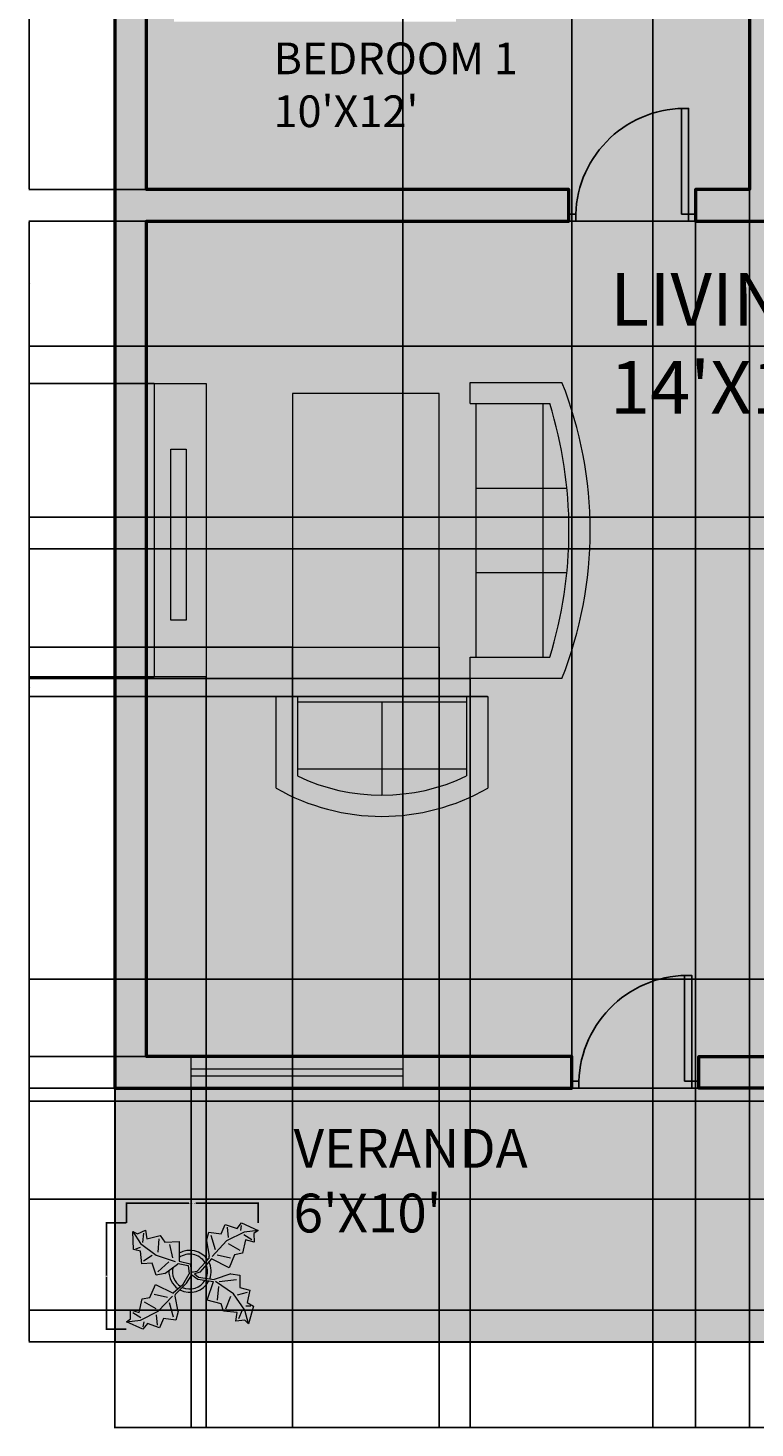
# Model space of a CAD drawing. Units: inches. Extents: x -494 to 1275, y 12 to 1194.
# Tile 1 of 8: x 87 to 293, y 346 to 743. Entities that reach past the tile are written whole.
import ezdxf

# ---------------------------------------------------------------- set-up
doc = ezdxf.new("R2010")
doc.units = ezdxf.units.IN
doc.header["$MEASUREMENT"] = 0
for name, color, linetype, lineweight in [('A-ANNO-DIMS', 2, 'Continuous', 18), ('A-AREA-IDEN', 7, 'Continuous', 25), ('A-DOOR', 3, 'Continuous', 25), ('A-DOOR-PATT', 7, 'Continuous', 13), ('A-FLOR', 7, 'Continuous', 30), ('A-FURN', 8, 'Continuous', 18), ('A-GLAZ', 4, 'Continuous', 18), ('A-GLAZ-FRAM-PATT', 7, 'Continuous', 13), ('A-GLAZ-GLAS-PATT', 4, 'Continuous', 13), ('A-WALL', 7, 'Continuous', 50), ('L-PLNT', 3, 'Continuous', 18)]:
    doc.layers.add(name, color=color, linetype=linetype, lineweight=lineweight)
for name, color, linetype, lineweight, true_color in [('A-FLOR-PATT', 51, 'Continuous', 13, 0xf8f6b0), ('A-FURN-PATT', 254, 'Continuous', 13, 0xfeeab9), ('A-WALL-PATT', 251, 'Continuous', 13, 0x636466)]:
    doc.layers.add(name, color=color, linetype=linetype, lineweight=lineweight, true_color=true_color)
doc.styles.get("Standard").update_dxf_attribs({"font": 'arial.ttf'})
doc.dimstyles.get("Standard").update_dxf_attribs({"dimtxt": 0.18, "dimasz": 0.18, "dimexe": 0.18, "dimexo": 0.0625, "dimgap": 0.09, "dimtad": 0, "dimtih": 1, "dimtoh": 1, "dimdec": 4, "dimzin": 0, "dimdsep": 46, "dimlunit": 4, "dimtxsty": 'Standard', "dimcen": 0.09, "dimadec": 0, "dimazin": 0, "dimtfac": 1, "dimtdec": 4, "dimtofl": 0, "dimtmove": 0, "dimatfit": 3, "dimfxl": 1, "dimtolj": 1, "dimtzin": 0, "dimarcsym": 0})

# ---------------------------------------------------------------- blocks, each defined once
blk = doc.blocks.new('Sofa - Roundback Loveseat 5 ft.')
for p, q in [((0, -32.44198), (0, -5.99998)), ((-24, -33.99998), (-24, -11.46958)), ((24.00004, -33.99998), (24.00004, -11.46958)), ((-23.9998, -13.38178), (23.99986, -13.38178)), ((-24, -32.44198), (24.00004, -32.44198))]:
    blk.add_line(p, q)
for points in [[(-24, -33.99998), (-30, -33.99998), (-30, -7.99998)], [(30.00004, -7.99998), (30.00004, -33.99998), (24.00004, -33.99998)]]:
    blk.add_lwpolyline(points)
for centre, radius, start, end in [((0, -60.24998), 60.24998, 60.13715, 119.8628), ((0, -61.38438), 55.38444, 64.32083, 115.6792)]:
    blk.add_arc(centre, radius, start, end)
blk = doc.blocks.new('WINDOW-60IN')
for p, q in [((3.5, 60), (3.5, 0)), ((5.5, 60), (5.5, 0))]:
    blk.add_line(p, q)
blk.add_lwpolyline([(9, 0), (0, 0), (0, 60), (9, 60)], close=True)
blk = doc.blocks.new('DOOR-SINGLE-36IN')
blk.add_lwpolyline([(34, 2, 0.414214), (2, 32), (4, 32), (4, 2), (2, 2), (2, 32)], format="xyb")
for points in [[(0, 0), (2, 0), (2, 2), (0, 2)], [(34, 0), (36, 0), (36, 2), (34, 2)]]:
    blk.add_lwpolyline(points, close=True)
blk = doc.blocks.new('PLANT-VERANDA')
h = blk.add_hatch(color=256)
h.dxf.hatch_style = 1
h.paths.add_polyline_path([(14.98, 24.96), (10.95, 24.77), (9.63, 26.57), (5.82, 25.7), (5.39, 28.16), (3.14, 27.06), (1.81, 27.74), (1.99, 22.6), (4, 22.14), (4.42, 18.56), (7.33, 18.76), (8.42, 15.4), (10.89, 15.82), (14.48, 18.48), (14.71, 18.7), (17.48, 18.06), (17.78, 15.71), (15.99, 12.65), (13.28, 10.22), (8.28, 12.71), (6.68, 9), (4.49, 8.6), (3.59, 4.8), (1.19, 5.49), (1.2, 2.99), (0, 2.09), (4.7, 0), (6, 1.6), (9.4, 0.41), (10.5, 3.11), (14, 2.62), (14.69, 5.02), (13.88, 9.42), (13.95, 9.99), (17.07, 13.11), (18.6, 15.45), (20.25, 14.18), (24.72, 13.6), (22.95, 8.3), (26.84, 7.24), (27.55, 5.12), (31.44, 4.77), (31.08, 2.29), (33.56, 2.64), (34.62, 1.58), (36.03, 6.53), (34.26, 7.59), (34.97, 11.13), (32.14, 11.84), (32.14, 15.37), (29.67, 15.73), (24.9, 14.15), (20.43, 14.8), (19.31, 15.71), (20.83, 16.24), (24.11, 19.95), (29.12, 17.46), (30.71, 21.17), (32.91, 21.57), (33.8, 25.37), (36.2, 24.68), (36.19, 27.18), (37.39, 28.08), (32.69, 30.17), (31.39, 28.57), (27.99, 29.76), (26.9, 27.06), (23.39, 27.55), (22.7, 25.15), (23.51, 20.75), (23.44, 20.18), (20.12, 16.5), (18.49, 16.24), (18.09, 18.58), (14.94, 19.37)])
h.paths.add_polyline_path([(14.94, 20.36), (14.94, 19.37), (18.09, 18.58), (18.49, 16.24), (20.12, 16.5), (22.33, 18.95, 0.422141)], flags=17)
h.paths.add_polyline_path([(17.78, 15.71), (17.48, 18.06), (14.71, 18.7), (14.48, 18.48), (13.15, 17.5, 0.320154), (15.44, 12.16), (15.99, 12.65)], flags=17)
h.paths.add_polyline_path([(22.35, 13.91), (20.25, 14.18), (18.6, 15.45), (17.07, 13.11), (15.85, 11.88, 0.365185)], flags=17)
h = blk.add_hatch(color=256)
h.dxf.hatch_style = 1
h.paths.add_polyline_path([(13.15, 17.5), (12.06, 16.69, 0.262498), (14.67, 11.47), (15.44, 12.16, -0.320272)])
h.paths.add_polyline_path([(14.95, 21.58), (14.94, 19.37), (18.09, 18.58), (18.49, 16.24), (20.12, 16.5), (23.05, 19.75, 0.39032)])
h = blk.add_hatch(color=256)
h.dxf.hatch_style = 1
h.paths.add_polyline_path([(22.65, 18.29), (20.83, 16.24), (19.31, 15.71), (20.43, 14.8), (22.64, 14.48, 0.196749)])
h.paths.add_polyline_path([(23.39, 19.14), (22.65, 18.29, -0.196749), (22.64, 14.48), (23.64, 14.33, 0.213013)])
h.paths.add_polyline_path([(23.41, 13.77), (20.25, 14.18), (18.6, 15.45), (17.07, 13.11), (15.15, 11.19, 0.412433)])
for p, q in [((3.14, 27.06), (5.39, 28.16)), ((5.39, 28.16), (5.82, 25.7)), ((26.9, 27.06), (27.99, 29.76)), ((27.99, 29.76), (31.39, 28.57)), ((28.59, 28.96), (28.9, 26.06)), ((31.39, 28.57), (32.69, 30.17)), ((32.59, 29.47), (32.39, 28.07)), ((32.69, 30.17), (37.39, 28.08)), ((37.39, 28.08), (33.39, 27.57)), ((37.39, 28.08), (36.19, 27.18)), ((1.81, 27.74), (4.02, 24.37)), ((1.81, 27.74), (3.14, 27.06)), ((1.99, 22.6), (1.81, 27.74)), ((4.02, 24.37), (8.46, 20.99)), ((4.69, 24.59), (4.93, 27.27)), ((5.82, 25.7), (9.63, 26.57)), ((9.17, 25.68), (8.92, 21.88)), ((9.63, 26.57), (10.95, 24.77)), ((10.95, 24.77), (14.98, 24.96)), ((13.16, 20.28), (12.29, 24.09)), ((14.98, 24.96), (14.94, 19.37)), ((22.7, 25.15), (23.39, 27.55)), ((22.7, 25.15), (23.51, 20.75)), ((23.39, 27.55), (26.9, 27.06)), ((24, 26.75), (25.21, 22.65)), ((28.4, 25.06), (24.29, 20.67)), ((33.39, 27.57), (28.4, 25.06)), ((32.31, 22.37), (29, 24.26)), ((33.8, 25.37), (32.91, 21.57)), ((33.3, 26.87), (35.6, 25.48)), ((36.2, 24.68), (33.8, 25.37)), ((36.19, 27.18), (36.2, 24.68)), ((4, 22.14), (1.99, 22.6)), ((2.66, 22.82), (4.01, 23.26)), ((4.42, 18.56), (4, 22.14)), ((4.88, 19.45), (7.35, 20.99)), ((8.46, 20.99), (13.82, 19.26)), ((20.12, 16.5), (23.44, 20.18)), ((24.11, 19.95), (20.83, 16.24)), ((23.44, 20.18), (23.51, 20.75)), ((29.12, 17.46), (24.11, 19.95)), ((25.71, 21.16), (29.51, 20.26)), ((30.71, 21.17), (29.12, 17.46)), ((32.91, 21.57), (30.71, 21.17)), ((7.33, 18.76), (4.42, 18.56)), ((8.42, 15.4), (7.33, 18.76)), ((8.88, 16.29), (12.03, 19.17)), ((10.89, 15.82), (14.48, 18.48)), ((14.48, 18.48), (14.71, 18.7)), ((14.71, 18.7), (17.48, 18.06)), ((14.94, 19.37), (18.09, 18.58)), ((17.48, 18.06), (17.78, 15.71)), ((17.48, 18.06), (17.48, 18.06)), ((18.09, 18.58), (18.49, 16.24)), ((18.49, 16.24), (20.12, 16.5)), ((20.83, 16.24), (19.31, 15.71)), ((6.68, 9), (8.28, 12.71)), ((8.28, 12.71), (13.28, 10.22)), ((10.89, 15.82), (8.42, 15.4)), ((15.99, 12.65), (13.28, 10.22)), ((13.95, 9.99), (17.07, 13.11)), ((15.99, 12.65), (17.78, 15.71)), ((17.07, 13.11), (18.6, 15.45)), ((18.6, 15.45), (20.25, 14.18)), ((19.31, 15.71), (20.43, 14.8)), ((20.25, 14.18), (24.72, 13.6)), ((20.43, 14.8), (24.9, 14.15)), ((22.95, 8.3), (24.72, 13.6)), ((29.67, 15.73), (24.9, 14.15)), ((30.38, 10.07), (25.23, 13.59)), ((26.13, 12.19), (25.78, 8.3)), ((26.36, 13.52), (31.21, 14.1)), ((29.67, 15.73), (32.14, 15.37)), ((32.14, 15.37), (32.14, 11.84)), ((3.59, 4.8), (4.49, 8.6)), ((4.49, 8.6), (6.68, 9)), ((11.68, 9.02), (7.88, 9.91)), ((8.99, 5.11), (13.1, 9.45)), ((13.88, 9.42), (13.95, 9.99)), ((14.69, 5.02), (13.88, 9.42)), ((26.84, 7.24), (22.95, 8.3)), ((28.25, 5.83), (29.67, 9.36)), ((33.56, 5.47), (30.38, 10.07)), ((34.26, 10.42), (31.44, 9.72)), ((32.14, 11.84), (34.97, 11.13)), ((34.97, 11.13), (34.26, 7.59)), ((1.19, 5.49), (3.59, 4.8)), ((1.2, 2.99), (1.19, 5.49)), ((4.1, 3.3), (1.79, 4.69)), ((4, 2.6), (8.99, 5.11)), ((5.09, 7.8), (8.39, 5.91)), ((8.8, 1.21), (8.5, 4.11)), ((13.4, 3.42), (12.19, 7.52)), ((14.69, 5.02), (14, 2.62)), ((27.55, 5.12), (26.84, 7.24)), ((31.44, 4.77), (27.55, 5.12)), ((31.08, 2.29), (31.44, 4.77)), ((32.85, 5.47), (31.79, 3)), ((34.62, 1.58), (33.56, 5.47)), ((35.33, 6.53), (33.91, 6.53)), ((34.26, 7.59), (36.03, 6.53)), ((36.03, 6.53), (34.62, 1.58)), ((0, 2.09), (1.2, 2.99)), ((0, 2.09), (4, 2.6)), ((4.7, 0), (0, 2.09)), ((6, 1.6), (4.7, 0)), ((4.8, 0.7), (5, 2.1)), ((9.4, 0.41), (6, 1.6)), ((10.5, 3.11), (9.4, 0.41)), ((14, 2.62), (10.5, 3.11)), ((33.56, 2.64), (31.08, 2.29)), ((34.62, 1.58), (33.56, 2.64))]:
    blk.add_line(p, q)
for centre, radius, start, end in [((18.01, 16.27), 6.13, 34.3757, 120.1028), ((17.95, 16.06), 5.25, 33.8219, 124.9414), ((18, 16.4), 5.94, 177.1741, 236.0068), ((18.04, 16.43), 5, 167.6804, 238.6774), ((17.99, 16.39), 5.03, 337.6469, 22.1698), ((18.14, 16.45), 5.9, 338.9388, 27.0389), ((17.98, 16.63), 6.14, 242.5292, 332.1842), ((17.9, 16.76), 5.29, 247.3711, 327.472)]:
    blk.add_arc(centre, radius, start, end)
blk = doc.blocks.new('SOFA-84IN-PLAN')
h = blk.add_hatch(color=256)
h.dxf.hatch_style = 1
h.paths.add_polyline_path([(20.62, 54), (1.56, 54), (1.56, 30), (20.62, 30)], flags=17)
h.paths.add_polyline_path([(20.62, 78), (1.56, 78), (1.56, 54), (20.62, 54)], flags=17)
h.paths.add_polyline_path([(22.53, 78), (20.62, 78), (20.62, 54), (27.4, 54, 0.050647)], flags=17)
h.paths.add_polyline_path([(27.4, 54), (20.62, 54), (20.62, 30), (27.4, 30, 0.049628)], flags=17)
h.paths.add_polyline_path([(20.62, 30), (1.56, 30), (1.56, 6), (20.62, 6)], flags=17)
h.paths.add_polyline_path([(27.4, 30), (20.62, 30), (20.62, 6), (22.53, 6, 0.050647)], flags=17)
h.paths.add_polyline_path([(26, 84), (0, 84), (0, 78), (22.53, 78, -0.050647), (27.4, 54, -0.100528), (22.53, 6), (20.62, 6), (1.56, 6), (0, 6), (0, 0), (26, 0, 0.190476)])
for p, q in [((0, 78), (22.53, 78)), ((1.56, 78), (1.56, 6)), ((20.62, 78), (20.62, 6)), ((1.56, 54), (27.4, 54)), ((1.56, 30), (27.4, 30)), ((0, 6), (22.53, 6))]:
    blk.add_line(p, q)
for points in [[(0, 78), (0, 84), (26, 84)], [(26, 0), (0, 0), (0, 6)]]:
    blk.add_lwpolyline(points)
for centre, radius, start, end in [((-80.25, 42), 114.25, 338.4314, 21.5686), ((-93.2, 42), 121.2, 342.7203, 17.2797)]:
    blk.add_arc(centre, radius, start, end)
blk = doc.blocks.new('TABLE-RECTANGULAR-72IN')
h = blk.add_hatch(color=256)
h.dxf.hatch_style = 1
h.paths.add_polyline_path([(41.56, 71.99), (0, 71.99), (0, 0), (41.56, 0)])
blk.add_lwpolyline([(0, 0), (41.56, 0), (41.56, 71.99), (0, 71.99)], close=True)
blk = doc.blocks.new('MEDIA-CONSOLE-PLAN')
for p, q in [((4.67, 64.59), (9.03, 64.59)), ((4.67, 16.07), (4.67, 64.59)), ((9.03, 64.59), (9.03, 16.07)), ((9.03, 16.07), (4.67, 16.07))]:
    blk.add_line(p, q)
blk.add_lwpolyline([(0, 83.25), (14.68, 83.25), (14.68, 0), (0, 0)], close=True)
blk = doc.blocks.new('*D30')
at = {"layer": 'A-ANNO-DIMS', "color": 0, "lineweight": -2, "transparency": 16777216}
for p, q in [((115.01, 404.34), (115.01, 410.07)), ((115.19, 409.89), (132.74, 409.89)), ((152.22, 409.89), (134.67, 409.89)), ((152.4, 404.34), (152.4, 410.07))]:
    blk.add_line(p, q, dxfattribs=at)
at = {"layer": 'A-ANNO-DIMS', "color": 0, "transparency": 16777216}
for points in [[(115.19, 409.92), (115.19, 409.86), (115.01, 409.89)], [(152.22, 409.92), (152.22, 409.86), (152.4, 409.89)]]:
    blk.add_solid(points, dxfattribs=at)
at = {"layer": 'Defpoints', "color": 0, "transparency": 16777216}
for p in [(152.4, 409.89), (115.01, 404.28), (152.4, 404.28)]:
    blk.add_point(p, dxfattribs=at)
at = {"layer": 'A-ANNO-DIMS', "color": 0, "transparency": 16777216, "insert": (133.7, 409.89), "char_height": 0.18, "attachment_point": 5}
blk.add_mtext('\\A1;PLANT 37 TYP.', dxfattribs=at)
blk = doc.blocks.new('*D31')
at = {"layer": 'A-ANNO-DIMS', "color": 0, "lineweight": -2, "transparency": 16777216}
for p, q in [((114.94, 404.28), (109.22, 404.28)), ((109.4, 404.1), (109.4, 389.38)), ((109.4, 374.29), (109.4, 389.01)), ((114.94, 374.11), (109.22, 374.11))]:
    blk.add_line(p, q, dxfattribs=at)
at = {"layer": 'A-ANNO-DIMS', "color": 0, "transparency": 16777216}
for points in [[(109.37, 404.1), (109.43, 404.1), (109.4, 404.28)], [(109.37, 374.29), (109.43, 374.29), (109.4, 374.11)]]:
    blk.add_solid(points, dxfattribs=at)
at = {"layer": 'Defpoints', "color": 0, "transparency": 16777216}
for p in [(109.4, 404.28), (115.01, 404.28), (115.01, 374.11)]:
    blk.add_point(p, dxfattribs=at)
at = {"layer": 'A-ANNO-DIMS', "color": 0, "transparency": 16777216, "insert": (109.4, 389.2), "char_height": 0.18, "attachment_point": 5}
blk.add_mtext('\\A1;30 TYP.', dxfattribs=at)
blk = doc.blocks.new('*D42')
at = {"layer": 'A-ANNO-DIMS', "color": 0, "lineweight": -2, "transparency": 16777216}
for p, q in [((111.73, 370.47), (111.73, 346.1)), ((471.73, 370.47), (471.73, 346.1)), ((111.91, 346.28), (291.44, 346.28)), ((471.55, 346.28), (292.02, 346.28))]:
    blk.add_line(p, q, dxfattribs=at)
at = {"layer": 'A-ANNO-DIMS', "color": 0, "transparency": 16777216}
for points in [[(111.91, 346.31), (111.91, 346.25), (111.73, 346.28)], [(471.55, 346.31), (471.55, 346.25), (471.73, 346.28)]]:
    blk.add_solid(points, dxfattribs=at)
at = {"layer": 'Defpoints', "color": 0, "transparency": 16777216}
for p in [(111.73, 370.53), (471.73, 370.53), (471.73, 346.28)]:
    blk.add_point(p, dxfattribs=at)
at = {"layer": 'A-ANNO-DIMS', "color": 0, "transparency": 16777216, "insert": (291.73, 346.28), "char_height": 0.18, "attachment_point": 5}
blk.add_mtext('\\A1;360', dxfattribs=at)
blk = doc.blocks.new('*D44')
at = {"layer": 'A-ANNO-DIMS', "color": 0, "lineweight": -2, "transparency": 16777216}
for p, q in [((111.67, 442.53), (87.3, 442.53)), ((87.48, 442.35), (87.48, 406.72)), ((87.48, 370.71), (87.48, 406.35)), ((111.67, 370.53), (87.3, 370.53))]:
    blk.add_line(p, q, dxfattribs=at)
at = {"layer": 'A-ANNO-DIMS', "color": 0, "transparency": 16777216}
for points in [[(87.45, 442.35), (87.51, 442.35), (87.48, 442.53)], [(87.45, 370.71), (87.51, 370.71), (87.48, 370.53)]]:
    blk.add_solid(points, dxfattribs=at)
at = {"layer": 'Defpoints', "color": 0, "transparency": 16777216}
for p in [(87.48, 442.53), (111.73, 442.53), (111.73, 370.53)]:
    blk.add_point(p, dxfattribs=at)
at = {"layer": 'A-ANNO-DIMS', "color": 0, "transparency": 16777216, "insert": (87.48, 406.53), "char_height": 0.18, "attachment_point": 5}
blk.add_mtext('\\A1;72', dxfattribs=at)
blk = doc.blocks.new('*D45')
at = {"layer": 'A-ANNO-DIMS', "color": 0, "lineweight": -2, "transparency": 16777216}
for p, q in [((120.67, 841.53), (87.3, 841.53)), ((87.48, 841.35), (87.48, 769.72)), ((87.48, 697.71), (87.48, 769.35)), ((120.67, 697.53), (87.3, 697.53))]:
    blk.add_line(p, q, dxfattribs=at)
at = {"layer": 'A-ANNO-DIMS', "color": 0, "transparency": 16777216}
for points in [[(87.45, 841.35), (87.51, 841.35), (87.48, 841.53)], [(87.45, 697.71), (87.51, 697.71), (87.48, 697.53)]]:
    blk.add_solid(points, dxfattribs=at)
at = {"layer": 'Defpoints', "color": 0, "transparency": 16777216}
for p in [(120.73, 841.53), (87.48, 697.53), (120.73, 697.53)]:
    blk.add_point(p, dxfattribs=at)
at = {"layer": 'A-ANNO-DIMS', "color": 0, "transparency": 16777216, "insert": (87.48, 769.53), "char_height": 0.18, "attachment_point": 5}
blk.add_mtext('\\A1;144', dxfattribs=at)
blk = doc.blocks.new('*D46')
at = {"layer": 'A-ANNO-DIMS', "color": 0, "lineweight": -2, "transparency": 16777216}
for p, q in [((120.67, 688.53), (87.3, 688.53)), ((87.48, 688.35), (87.48, 570.22)), ((87.48, 451.71), (87.48, 569.85)), ((120.67, 451.53), (87.3, 451.53))]:
    blk.add_line(p, q, dxfattribs=at)
at = {"layer": 'A-ANNO-DIMS', "color": 0, "transparency": 16777216}
for points in [[(87.45, 688.35), (87.51, 688.35), (87.48, 688.53)], [(87.45, 451.71), (87.51, 451.71), (87.48, 451.53)]]:
    blk.add_solid(points, dxfattribs=at)
at = {"layer": 'Defpoints', "color": 0, "transparency": 16777216}
for p in [(87.48, 688.53), (120.73, 688.53), (120.73, 451.53)]:
    blk.add_point(p, dxfattribs=at)
at = {"layer": 'A-ANNO-DIMS', "color": 0, "transparency": 16777216, "insert": (87.48, 570.03), "char_height": 0.18, "attachment_point": 5}
blk.add_mtext('\\A1;237', dxfattribs=at)
blk = doc.blocks.new('*D51')
at = {"layer": 'A-ANNO-DIMS', "color": 0, "lineweight": -2, "transparency": 16777216}
for p, q in [((111.73, 442.47), (111.73, 346.1)), ((133.38, 442.47), (133.38, 346.1)), ((111.91, 346.28), (122.09, 346.28)), ((133.2, 346.28), (123.02, 346.28))]:
    blk.add_line(p, q, dxfattribs=at)
at = {"layer": 'A-ANNO-DIMS', "color": 0, "transparency": 16777216}
for points in [[(111.91, 346.31), (111.91, 346.25), (111.73, 346.28)], [(133.2, 346.31), (133.2, 346.25), (133.38, 346.28)]]:
    blk.add_solid(points, dxfattribs=at)
at = {"layer": 'Defpoints', "color": 0, "transparency": 16777216}
for p in [(111.73, 442.53), (133.38, 442.53), (133.38, 346.28)]:
    blk.add_point(p, dxfattribs=at)
at = {"layer": 'A-ANNO-DIMS', "color": 0, "transparency": 16777216, "insert": (122.56, 346.28), "char_height": 0.18, "attachment_point": 5}
blk.add_mtext('\\A1;21.646', dxfattribs=at)
blk = doc.blocks.new('*D52')
at = {"layer": 'A-ANNO-DIMS', "color": 0, "lineweight": -2, "transparency": 16777216}
for p, q in [((193.38, 451.6), (193.38, 874.96)), ((193.56, 874.78), (216.96, 874.78)), ((241.16, 874.78), (217.76, 874.78)), ((241.34, 451.6), (241.34, 874.96))]:
    blk.add_line(p, q, dxfattribs=at)
at = {"layer": 'A-ANNO-DIMS', "color": 0, "transparency": 16777216}
for points in [[(193.56, 874.81), (193.56, 874.75), (193.38, 874.78)], [(241.16, 874.81), (241.16, 874.75), (241.34, 874.78)]]:
    blk.add_solid(points, dxfattribs=at)
at = {"layer": 'Defpoints', "color": 0, "transparency": 16777216}
for p in [(241.34, 874.78), (193.38, 451.53), (241.34, 451.53)]:
    blk.add_point(p, dxfattribs=at)
at = {"layer": 'A-ANNO-DIMS', "color": 0, "transparency": 16777216, "insert": (217.36, 874.78), "char_height": 0.18, "attachment_point": 5}
blk.add_mtext('\\A1;47.96', dxfattribs=at)
blk = doc.blocks.new('*D54')
at = {"layer": 'A-ANNO-DIMS', "color": 0, "lineweight": -2, "transparency": 16777216}
for p, q in [((291.73, 697.47), (291.73, 346.1)), ((276.46, 688.47), (276.46, 346.1)), ((276.64, 346.28), (283.64, 346.28)), ((291.55, 346.28), (284.55, 346.28))]:
    blk.add_line(p, q, dxfattribs=at)
at = {"layer": 'A-ANNO-DIMS', "color": 0, "transparency": 16777216}
for points in [[(276.64, 346.31), (276.64, 346.25), (276.46, 346.28)], [(291.55, 346.31), (291.55, 346.25), (291.73, 346.28)]]:
    blk.add_solid(points, dxfattribs=at)
at = {"layer": 'Defpoints', "color": 0, "transparency": 16777216}
for p in [(291.73, 697.53), (276.46, 688.53), (291.73, 346.28)]:
    blk.add_point(p, dxfattribs=at)
at = {"layer": 'A-ANNO-DIMS', "color": 0, "transparency": 16777216, "insert": (284.09, 346.28), "char_height": 0.18, "attachment_point": 5}
blk.add_mtext('\\A1;15.276', dxfattribs=at)
blk = doc.blocks.new('*D55')
at = {"layer": 'A-ANNO-DIMS', "color": 0, "lineweight": -2, "transparency": 16777216}
for p, q in [((402.67, 688.53), (87.3, 688.53)), ((87.48, 688.35), (87.48, 646.72)), ((87.48, 604.71), (87.48, 646.35)), ((402.67, 604.53), (87.3, 604.53))]:
    blk.add_line(p, q, dxfattribs=at)
at = {"layer": 'A-ANNO-DIMS', "color": 0, "transparency": 16777216}
for points in [[(87.45, 688.35), (87.51, 688.35), (87.48, 688.53)], [(87.45, 604.71), (87.51, 604.71), (87.48, 604.53)]]:
    blk.add_solid(points, dxfattribs=at)
at = {"layer": 'Defpoints', "color": 0, "transparency": 16777216}
for p in [(87.48, 688.53), (402.73, 688.53), (402.73, 604.53)]:
    blk.add_point(p, dxfattribs=at)
at = {"layer": 'A-ANNO-DIMS', "color": 0, "transparency": 16777216, "insert": (87.48, 646.53), "char_height": 0.18, "attachment_point": 5}
blk.add_mtext('\\A1;84', dxfattribs=at)
blk = doc.blocks.new('*D59')
at = {"layer": 'A-ANNO-DIMS', "color": 0, "lineweight": -2, "transparency": 16777216}
for p, q in [((342.67, 473.5), (87.3, 473.5)), ((87.48, 473.32), (87.48, 426.7)), ((87.48, 379.71), (87.48, 426.33)), ((342.67, 379.53), (87.3, 379.53))]:
    blk.add_line(p, q, dxfattribs=at)
at = {"layer": 'A-ANNO-DIMS', "color": 0, "transparency": 16777216}
for points in [[(87.45, 473.32), (87.51, 473.32), (87.48, 473.5)], [(87.45, 379.71), (87.51, 379.71), (87.48, 379.53)]]:
    blk.add_solid(points, dxfattribs=at)
at = {"layer": 'Defpoints', "color": 0, "transparency": 16777216}
for p in [(87.48, 473.5), (342.73, 473.5), (342.73, 379.53)]:
    blk.add_point(p, dxfattribs=at)
at = {"layer": 'A-ANNO-DIMS', "color": 0, "transparency": 16777216, "insert": (87.48, 426.52), "char_height": 0.18, "attachment_point": 5}
blk.add_mtext('\\A1;93.96', dxfattribs=at)
blk = doc.blocks.new('*D61')
at = {"layer": 'A-ANNO-DIMS', "color": 0, "lineweight": -2, "transparency": 16777216}
for p, q in [((393.67, 688.53), (87.3, 688.53)), ((87.48, 688.35), (87.48, 671.01)), ((87.48, 653.3), (87.48, 670.64)), ((393.67, 653.12), (87.3, 653.12))]:
    blk.add_line(p, q, dxfattribs=at)
at = {"layer": 'A-ANNO-DIMS', "color": 0, "transparency": 16777216}
for points in [[(87.45, 688.35), (87.51, 688.35), (87.48, 688.53)], [(87.45, 653.3), (87.51, 653.3), (87.48, 653.12)]]:
    blk.add_solid(points, dxfattribs=at)
at = {"layer": 'Defpoints', "color": 0, "transparency": 16777216}
for p in [(393.73, 688.53), (87.48, 653.12), (393.73, 653.12)]:
    blk.add_point(p, dxfattribs=at)
at = {"layer": 'A-ANNO-DIMS', "color": 0, "transparency": 16777216, "insert": (87.48, 670.83), "char_height": 0.18, "attachment_point": 5}
blk.add_mtext('\\A1;35.416', dxfattribs=at)
blk = doc.blocks.new('*D63')
at = {"layer": 'A-ANNO-DIMS', "color": 0, "lineweight": -2, "transparency": 16777216}
for p, q in [((402.67, 595.53), (87.3, 595.53)), ((87.48, 595.35), (87.48, 487.72)), ((87.48, 379.71), (87.48, 487.35)), ((342.67, 379.53), (87.3, 379.53))]:
    blk.add_line(p, q, dxfattribs=at)
at = {"layer": 'A-ANNO-DIMS', "color": 0, "transparency": 16777216}
for points in [[(87.45, 595.35), (87.51, 595.35), (87.48, 595.53)], [(87.45, 379.71), (87.51, 379.71), (87.48, 379.53)]]:
    blk.add_solid(points, dxfattribs=at)
at = {"layer": 'Defpoints', "color": 0, "transparency": 16777216}
for p in [(402.73, 595.53), (87.48, 379.53), (342.73, 379.53)]:
    blk.add_point(p, dxfattribs=at)
at = {"layer": 'A-ANNO-DIMS', "color": 0, "transparency": 16777216, "insert": (87.48, 487.53), "char_height": 0.18, "attachment_point": 5}
blk.add_mtext('\\A1;216', dxfattribs=at)
blk = doc.blocks.new('*D68')
at = {"layer": 'A-ANNO-DIMS', "color": 0, "lineweight": -2, "transparency": 16777216}
for p, q in [((458.91, 438.82), (87.3, 438.82)), ((87.48, 438.64), (87.48, 409.36)), ((87.48, 379.71), (87.48, 408.99)), ((462.68, 379.53), (87.3, 379.53))]:
    blk.add_line(p, q, dxfattribs=at)
at = {"layer": 'A-ANNO-DIMS', "color": 0, "transparency": 16777216}
for points in [[(87.45, 438.64), (87.51, 438.64), (87.48, 438.82)], [(87.45, 379.71), (87.51, 379.71), (87.48, 379.53)]]:
    blk.add_solid(points, dxfattribs=at)
at = {"layer": 'Defpoints', "color": 0, "transparency": 16777216}
for p in [(87.48, 438.82), (458.98, 438.82), (462.74, 379.53)]:
    blk.add_point(p, dxfattribs=at)
at = {"layer": 'A-ANNO-DIMS', "color": 0, "transparency": 16777216, "insert": (87.48, 409.18), "char_height": 0.18, "attachment_point": 5}
blk.add_mtext('\\A1;59.28', dxfattribs=at)
blk = doc.blocks.new('*D82')
at = {"layer": 'A-ANNO-DIMS', "color": 0, "lineweight": -2, "transparency": 16777216}
for p, q in [((264.34, 820.48), (264.34, 346.1)), ((291.73, 820.48), (291.73, 346.1)), ((264.52, 346.28), (277.57, 346.28)), ((291.55, 346.28), (278.5, 346.28))]:
    blk.add_line(p, q, dxfattribs=at)
at = {"layer": 'A-ANNO-DIMS', "color": 0, "transparency": 16777216}
for points in [[(264.52, 346.31), (264.52, 346.25), (264.34, 346.28)], [(291.55, 346.31), (291.55, 346.25), (291.73, 346.28)]]:
    blk.add_solid(points, dxfattribs=at)
at = {"layer": 'Defpoints', "color": 0, "transparency": 16777216}
for p in [(264.34, 820.54), (291.73, 820.54), (291.73, 346.28)]:
    blk.add_point(p, dxfattribs=at)
at = {"layer": 'A-ANNO-DIMS', "color": 0, "transparency": 16777216, "insert": (278.04, 346.28), "char_height": 0.18, "attachment_point": 5}
blk.add_mtext('\\A1;27.394', dxfattribs=at)
blk = doc.blocks.new('*D86')
at = {"layer": 'A-ANNO-DIMS', "color": 0, "lineweight": -2, "transparency": 16777216}
for p, q in [((120.67, 688.53), (87.3, 688.53)), ((87.48, 688.35), (87.48, 665.71)), ((87.48, 642.7), (87.48, 665.34)), ((122.89, 642.52), (87.3, 642.52))]:
    blk.add_line(p, q, dxfattribs=at)
at = {"layer": 'A-ANNO-DIMS', "color": 0, "transparency": 16777216}
for points in [[(87.45, 688.35), (87.51, 688.35), (87.48, 688.53)], [(87.45, 642.7), (87.51, 642.7), (87.48, 642.52)]]:
    blk.add_solid(points, dxfattribs=at)
at = {"layer": 'Defpoints', "color": 0, "transparency": 16777216}
for p in [(120.73, 688.53), (87.48, 642.52), (122.96, 642.52)]:
    blk.add_point(p, dxfattribs=at)
at = {"layer": 'A-ANNO-DIMS', "color": 0, "transparency": 16777216, "insert": (87.48, 665.53), "char_height": 0.18, "attachment_point": 5}
blk.add_mtext('\\A1;46.02', dxfattribs=at)
blk = doc.blocks.new('*D87')
at = {"layer": 'A-ANNO-DIMS', "color": 0, "lineweight": -2, "transparency": 16777216}
for p, q in [((162.13, 567.63), (162.13, 346.1)), ((137.63, 559.21), (137.63, 346.1)), ((137.81, 346.28), (149.48, 346.28)), ((161.95, 346.28), (150.28, 346.28))]:
    blk.add_line(p, q, dxfattribs=at)
at = {"layer": 'A-ANNO-DIMS', "color": 0, "transparency": 16777216}
for points in [[(137.81, 346.31), (137.81, 346.25), (137.63, 346.28)], [(161.95, 346.31), (161.95, 346.25), (162.13, 346.28)]]:
    blk.add_solid(points, dxfattribs=at)
at = {"layer": 'Defpoints', "color": 0, "transparency": 16777216}
for p in [(162.13, 567.7), (137.63, 559.27), (162.13, 346.28)]:
    blk.add_point(p, dxfattribs=at)
at = {"layer": 'A-ANNO-DIMS', "color": 0, "transparency": 16777216, "insert": (149.88, 346.28), "char_height": 0.18, "attachment_point": 5}
blk.add_mtext('\\A1;24.49', dxfattribs=at)
blk = doc.blocks.new('*D88')
at = {"layer": 'A-ANNO-DIMS', "color": 0, "lineweight": -2, "transparency": 16777216}
for p, q in [((203.69, 567.63), (203.69, 346.1)), ((212.54, 558.75), (212.54, 346.1)), ((203.87, 346.28), (207.72, 346.28)), ((212.36, 346.28), (208.51, 346.28))]:
    blk.add_line(p, q, dxfattribs=at)
at = {"layer": 'A-ANNO-DIMS', "color": 0, "transparency": 16777216}
for points in [[(203.87, 346.31), (203.87, 346.25), (203.69, 346.28)], [(212.36, 346.31), (212.36, 346.25), (212.54, 346.28)]]:
    blk.add_solid(points, dxfattribs=at)
at = {"layer": 'Defpoints', "color": 0, "transparency": 16777216}
for p in [(203.69, 567.7), (212.54, 558.81), (212.54, 346.28)]:
    blk.add_point(p, dxfattribs=at)
at = {"layer": 'A-ANNO-DIMS', "color": 0, "transparency": 16777216, "insert": (208.12, 346.28), "char_height": 0.18, "attachment_point": 5}
blk.add_mtext('\\A1;8.855', dxfattribs=at)
blk = doc.blocks.new('*D89')
at = {"layer": 'A-ANNO-DIMS', "color": 0, "lineweight": -2, "transparency": 16777216}
for p, q in [((212.48, 558.81), (87.3, 558.81)), ((87.48, 558.63), (87.48, 556.42)), ((217.43, 553.67), (87.3, 553.67)), ((87.48, 553.85), (87.48, 556.06))]:
    blk.add_line(p, q, dxfattribs=at)
at = {"layer": 'A-ANNO-DIMS', "color": 0, "transparency": 16777216}
for points in [[(87.45, 558.63), (87.51, 558.63), (87.48, 558.81)], [(87.45, 553.85), (87.51, 553.85), (87.48, 553.67)]]:
    blk.add_solid(points, dxfattribs=at)
at = {"layer": 'Defpoints', "color": 0, "transparency": 16777216}
for p in [(212.54, 558.81), (87.48, 553.67), (217.49, 553.67)]:
    blk.add_point(p, dxfattribs=at)
at = {"layer": 'A-ANNO-DIMS', "color": 0, "transparency": 16777216, "insert": (87.48, 556.24), "char_height": 0.18, "attachment_point": 5}
blk.add_mtext('\\A1;5.145', dxfattribs=at)
blk = doc.blocks.new('*D90')
at = {"layer": 'A-ANNO-DIMS', "color": 0, "lineweight": -2, "transparency": 16777216}
for p, q in [((162.06, 567.7), (87.3, 567.7)), ((87.48, 567.52), (87.48, 563.67)), ((87.48, 559.45), (87.48, 563.3)), ((122.89, 559.27), (87.3, 559.27))]:
    blk.add_line(p, q, dxfattribs=at)
at = {"layer": 'A-ANNO-DIMS', "color": 0, "transparency": 16777216}
for points in [[(87.45, 567.52), (87.51, 567.52), (87.48, 567.7)], [(87.45, 559.45), (87.51, 559.45), (87.48, 559.27)]]:
    blk.add_solid(points, dxfattribs=at)
at = {"layer": 'Defpoints', "color": 0, "transparency": 16777216}
for p in [(162.13, 567.7), (87.48, 559.27), (122.96, 559.27)]:
    blk.add_point(p, dxfattribs=at)
at = {"layer": 'A-ANNO-DIMS', "color": 0, "transparency": 16777216, "insert": (87.48, 563.48), "char_height": 0.18, "attachment_point": 5}
blk.add_mtext('\\A1;8.426', dxfattribs=at)
blk = doc.blocks.new('*D97')
at = {"layer": 'A-ANNO-DIMS', "color": 0, "lineweight": -2, "transparency": 16777216}
for p, q in [((342.67, 411.03), (87.3, 411.03)), ((87.48, 410.85), (87.48, 395.47)), ((87.48, 379.71), (87.48, 395.1)), ((342.67, 379.53), (87.3, 379.53))]:
    blk.add_line(p, q, dxfattribs=at)
at = {"layer": 'A-ANNO-DIMS', "color": 0, "transparency": 16777216}
for points in [[(87.45, 410.85), (87.51, 410.85), (87.48, 411.03)], [(87.45, 379.71), (87.51, 379.71), (87.48, 379.53)]]:
    blk.add_solid(points, dxfattribs=at)
at = {"layer": 'Defpoints', "color": 0, "transparency": 16777216}
for p in [(342.73, 411.03), (87.48, 379.53), (342.73, 379.53)]:
    blk.add_point(p, dxfattribs=at)
at = {"layer": 'A-ANNO-DIMS', "color": 0, "transparency": 16777216, "insert": (87.48, 395.28), "char_height": 0.18, "attachment_point": 5}
blk.add_mtext('\\A1;31.5', dxfattribs=at)

msp = doc.modelspace()

# ---------------------------------------------------------------- hatches: boundary and pattern name
at = {"layer": 'A-DOOR-PATT'}
h = msp.add_hatch(color=256, dxfattribs=at)
h.dxf.hatch_style = 1
h.paths.add_polyline_path([(274.4565, 720.5349), (272.4565, 720.5349), (272.4565, 690.5349), (274.4565, 690.5349)])
h.paths.add_polyline_path([(276.4565, 688.5349), (276.4565, 690.5349), (274.4565, 690.5349), (274.4565, 688.5349)])
h.paths.add_polyline_path([(240.4565, 688.5349), (242.4565, 688.5349), (242.4565, 690.5349), (240.4565, 690.5349)])
h = msp.add_hatch(color=256, dxfattribs=at)
h.dxf.hatch_style = 1
h.paths.add_polyline_path([(275.3385, 474.5349), (273.3385, 474.5349), (273.3385, 444.5349), (275.3385, 444.5349)])
h.paths.add_polyline_path([(277.3385, 442.5349), (277.3385, 444.5349), (275.3385, 444.5349), (275.3385, 442.5349)])
h.paths.add_polyline_path([(241.3385, 442.5349), (243.3385, 442.5349), (243.3385, 444.5349), (241.3385, 444.5349)])
at = {"layer": 'A-FLOR-PATT'}
h = msp.add_hatch(color=256, dxfattribs=at)
h.dxf.hatch_style = 1
h.paths.add_polyline_path([(333.7322, 595.5349), (393.7322, 595.5349), (393.7322, 617.1185), (393.7322, 653.1185), (393.7322, 688.5349), (348.3096, 688.5349), (348.3096, 697.5349), (462.7322, 697.5349), (462.7322, 841.5349), (300.7322, 841.5349), (300.7322, 820.5433), (323.2889, 820.5433), (323.2889, 769.5349), (300.7322, 769.5349), (300.7322, 697.5349), (312.3096, 697.5349), (312.3096, 688.5349), (276.4565, 688.5349), (276.4565, 697.5349), (291.7322, 697.5349), (291.7322, 771.5415), (264.338, 771.5415), (264.338, 820.5433), (291.7322, 820.5433), (291.7322, 841.5349), (120.7322, 841.5349), (120.7322, 697.5349), (240.4565, 697.5349), (240.4565, 688.5349), (120.7322, 688.5349), (120.7322, 451.5349), (241.3385, 451.5349), (241.3385, 442.5349), (277.3385, 442.5349), (277.3385, 451.5349), (333.7322, 451.5349), (333.7322, 473.4986), (333.7322, 509.4986)])
h.paths.add_polyline_path([(372.4977, 745.1275), (372.4977, 805.1275), (452.4977, 805.1275), (452.4977, 745.1275)], flags=16)
h.paths.add_polyline_path([(208.4976, 745.1275), (128.4976, 745.1275), (128.4976, 805.1275), (208.4976, 805.1275)], flags=16)
h.paths.add_polyline_path([(422.8977, 745.1275), (422.8977, 760.3275), (438.0977, 760.3275), (438.0977, 797.1275), (451.2977, 797.1275), (451.2977, 776.3275), (438.0977, 776.3275), (438.0977, 773.9275), (451.2977, 773.9275), (451.2977, 753.1275), (436.0977, 753.1275), (436.0977, 758.3275)], flags=16)
h.paths.add_polyline_path([(142.8976, 789.9275), (142.8976, 753.1275), (129.6976, 753.1275), (129.6976, 773.9275), (142.8976, 773.9275), (142.8976, 776.3275), (129.6976, 776.3275), (129.6976, 797.1275), (144.8976, 797.1275), (144.8976, 791.9275), (158.0976, 805.1275), (158.0976, 789.9275)], flags=0)
h = msp.add_hatch(color=256, dxfattribs=at)
h.dxf.hatch_style = 1
h.paths.add_polyline_path([(333.7322, 442.5349), (277.3385, 442.5349), (241.3385, 442.5349), (111.7322, 442.5349), (111.7322, 370.5349), (333.7322, 370.5349)])
at = {"layer": 'A-FURN-PATT'}
h = msp.add_hatch(color=256, dxfattribs=at)
h.dxf.hatch_style = 1
h.paths.add_polyline_path([(137.6337, 642.5177), (122.955, 642.5177), (122.955, 559.2709), (137.6337, 559.2709)])
h.paths.add_polyline_path([(127.6266, 575.3426), (127.6266, 623.8611), (131.9861, 623.8611), (131.9861, 575.3426)], flags=16)
h = msp.add_hatch(color=256, dxfattribs=at)
h.dxf.hatch_style = 1
h.paths.add_polyline_path([(131.9861, 623.8611), (127.6266, 623.8611), (127.6266, 575.3426), (131.9861, 575.3426)])
h = msp.add_hatch(color=256, dxfattribs=at)
h.dxf.hatch_style = 1
h.paths.add_polyline_path([(211.4947, 552.1079), (187.4947, 552.1079), (187.4947, 533.0477), (211.4947, 533.0477)], flags=17)
h.paths.add_polyline_path([(163.4946, 552.1079), (163.4946, 533.0477), (187.4947, 533.0477), (187.4947, 552.1079)], flags=17)
h.paths.add_polyline_path([(187.4947, 525.6658), (187.4947, 533.0477), (163.4946, 533.0477), (163.4946, 531.136, 0.11251889)], flags=16)
h.paths.add_polyline_path([(211.4947, 531.136), (211.4947, 533.0477), (187.4947, 533.0477), (187.4947, 525.6658, 0.11251869)], flags=17)
h.paths.add_polyline_path([(163.4946, 531.136), (163.4946, 553.6659), (157.4946, 553.6659), (157.4946, 527.6659, 0.26666697), (217.4947, 527.6659), (217.4947, 553.6659), (211.4947, 553.6659), (211.4947, 531.136, -0.22792319)])
at = {"layer": 'A-GLAZ-FRAM-PATT'}
h = msp.add_hatch(color=256, dxfattribs=at)
h.dxf.hatch_style = 1
h.paths.add_polyline_path([(193.3783, 451.5349), (133.3783, 451.5349), (133.3783, 448.0349), (193.3783, 448.0349)])
h.paths.add_polyline_path([(193.3783, 446.0349), (133.3783, 446.0349), (133.3783, 442.5349), (193.3783, 442.5349)])
at = {"layer": 'A-GLAZ-GLAS-PATT'}
h = msp.add_hatch(color=256, dxfattribs=at)
h.dxf.hatch_style = 1
h.paths.add_polyline_path([(193.3783, 448.0349), (133.3783, 448.0349), (133.3783, 446.0349), (193.3783, 446.0349)])
at = {"layer": 'A-WALL-PATT'}
h = msp.add_hatch(color=256, dxfattribs=at)
h.dxf.hatch_style = 1
h.paths.add_polyline_path([(120.7322, 841.5349), (291.7322, 841.5349), (291.7322, 697.5349), (276.4565, 697.5349), (276.4565, 688.5349), (312.3096, 688.5349), (312.3096, 697.5349), (300.7322, 697.5349), (300.7322, 841.5349), (462.7322, 841.5349), (462.7322, 697.5349), (348.3096, 697.5349), (348.3096, 688.5349), (393.7322, 688.5349), (393.7322, 653.1185), (402.7322, 653.1185), (402.7322, 688.5349), (462.7322, 688.5349), (462.7322, 604.5349), (402.7322, 604.5349), (402.7322, 617.1185), (393.7322, 617.1185), (393.7322, 595.5349), (333.7322, 595.5349), (333.7322, 509.4986), (342.7322, 509.4986), (342.7322, 586.5349), (393.7322, 586.5349), (402.7322, 586.5349), (402.7322, 595.5349), (462.9409, 595.5349), (462.7406, 379.5349), (342.7322, 379.5349), (342.7322, 442.5349), (342.7322, 473.4986), (333.7322, 473.4986), (333.7322, 451.5349), (277.3385, 451.5349), (277.3385, 442.5349), (333.7322, 442.5349), (333.7322, 370.5349), (471.7322, 370.5349), (471.7322, 850.5349), (111.7322, 850.5349), (111.7322, 442.5349), (241.3385, 442.5349), (241.3385, 451.5349), (120.7322, 451.5349), (120.7322, 688.5349), (240.4565, 688.5349), (240.4565, 697.5349), (120.7322, 697.5349)])

# ---------------------------------------------------------------- linework, layer by layer
at = {"layer": 'A-DOOR'}
msp.add_line((241.3385, 442.5349), (277.3385, 442.5349), dxfattribs=at)
msp.add_lwpolyline([(274.4565, 688.5349), (276.4565, 688.5349), (276.4565, 690.5349), (274.4565, 690.5349)], close=True, dxfattribs=at)
at = {"layer": 'A-FLOR'}
for p, q in [((111.7322, 442.5349), (111.7322, 370.5349)), ((111.7322, 370.5349), (333.7322, 370.5349))]:
    msp.add_line(p, q, dxfattribs=at)
at = {"layer": 'A-WALL'}
for points in [[(333.7322, 442.5349), (333.7322, 370.5349), (471.7322, 370.5349), (471.7322, 850.5349), (111.7322, 850.5349), (111.7322, 442.5349), (241.3385, 442.5349), (241.3385, 451.5349), (120.7322, 451.5349), (120.7322, 688.5349), (240.4565, 688.5349), (240.4565, 697.5349), (120.7322, 697.5349), (120.7322, 841.5349), (291.7322, 841.5349), (291.7322, 697.5349), (276.4565, 697.5349), (276.4565, 688.5349), (312.3096, 688.5349), (312.3096, 697.5349), (300.7322, 697.5349), (300.7322, 841.5349)], [(333.7322, 442.5349), (277.3385, 442.5349), (277.3385, 451.5349), (333.7322, 451.5349), (333.7322, 473.4986), (342.7322, 473.4986), (342.7322, 442.5349), (342.7322, 379.5349), (462.7406, 379.5349), (462.9409, 595.5349)]]:
    msp.add_lwpolyline(points, dxfattribs=at)

# ---------------------------------------------------------------- block references
at = {"layer": 'A-DOOR', "extrusion": (0, 0, -1), "zscale": -1}
for p in [(-276.4562, 688.535), (-277.3381, 442.535)]:
    msp.add_blockref('DOOR-SINGLE-36IN', p, dxfattribs=at)
at = {"layer": 'A-FURN'}
for name, p in [('MEDIA-CONSOLE-PLAN', (122.9554, 559.2708)), ('TABLE-RECTANGULAR-72IN', (162.1261, 567.6966)), ('SOFA-84IN-PLAN', (212.5452, 558.8108))]:
    msp.add_blockref(name, p, dxfattribs=at)
at = {"layer": 'A-FURN', "rotation": 180}
msp.add_blockref('Sofa - Roundback Loveseat 5 ft.', (187.4947, 519.6659), dxfattribs=at)
at = {"layer": 'A-GLAZ', "rotation": 90.00000000000026}
msp.add_blockref('WINDOW-60IN', (193.3778, 442.5346), dxfattribs=at)
at = {"layer": 'L-PLNT'}
msp.add_blockref('PLANT-VERANDA', (115.007, 374.11), dxfattribs=at)

# ---------------------------------------------------------------- texts
at = {"layer": 'A-AREA-IDEN', "attachment_point": 1}
for s, width, insert, char_height in [("BEDROOM 1\\P10'X12'", 73.167157, (156.7362, 739.2331), 9), ("LIVING/HALL\\P14'X16'", 130.54611, (252.1968, 673.8839), 15), ("VERANDA\\P6'X10'", 116.658127, (162.4375, 430.94), 11)]:
    msp.add_mtext_dynamic_manual_height_columns(s, width=width, gutter_width=1, heights=[0], dxfattribs=dict(at, insert=insert, char_height=char_height))

# ---------------------------------------------------------------- dimensions: what is measured, and where the dimension line sits
at = {"layer": 'A-ANNO-DIMS'}
for base, p1, p2, override, picture, middle in [((241.3385, 874.7849), (193.3783, 451.5349), (241.3385, 451.5349), {"dimdec": 2, "dimlfac": 1, "dimrnd": 0, "dimzin": 0, "dimdsep": 46, "dimlunit": 2}, '*D52', (217.3584, 874.7849)), ((291.7322, 346.2849), (264.338, 820.5433), (291.7322, 820.5433), {"dimdec": 3, "dimlfac": 1, "dimrnd": 0, "dimzin": 0, "dimdsep": 46, "dimlunit": 2}, '*D82', (278.0351, 346.2849)), ((291.7322, 346.2849), (276.4565, 688.5349), (291.7322, 697.5349), {"dimdec": 3, "dimlfac": 1, "dimrnd": 0, "dimzin": 0, "dimdsep": 46, "dimlunit": 2}, '*D54', (284.0944, 346.2849)), ((162.1259, 346.2849), (137.6337, 559.2709), (162.1259, 567.6964), {"dimdec": 2, "dimlfac": 1, "dimrnd": 0, "dimzin": 0, "dimdsep": 46, "dimlunit": 2}, '*D87', (149.8798, 346.2849)), ((212.5449, 346.2849), (203.6898, 567.6964), (212.5449, 558.8107), {"dimdec": 3, "dimlfac": 1, "dimrnd": 0, "dimzin": 0, "dimdsep": 46, "dimlunit": 2}, '*D88', (208.1173, 346.2849)), ((133.3783, 346.2849), (111.7322, 442.5349), (133.3783, 442.5349), {"dimdec": 3, "dimlfac": 1, "dimrnd": 0, "dimzin": 0, "dimdsep": 46, "dimlunit": 2}, '*D51', (122.5552, 346.2849)), ((471.7322, 346.2849), (111.7322, 370.5349), (471.7322, 370.5349), {"dimdec": 0, "dimlfac": 1, "dimrnd": 0, "dimzin": 0, "dimdsep": 46, "dimlunit": 2}, '*D42', (291.7322, 346.2849))]:
    dim = msp.add_linear_dim(base=base, p1=p1, p2=p2, dimstyle='Standard', override=override, dxfattribs=at)
    dim.commit()
    dim.dimension.update_dxf_attribs({"geometry": picture, "text_midpoint": middle})
for base, p1, p2, override, picture, middle in [((87.4822, 697.5349), (120.7322, 841.5349), (120.7322, 697.5349), {"dimdec": 0, "dimlfac": 1, "dimrnd": 0, "dimzin": 0, "dimdsep": 46, "dimlunit": 2}, '*D45', (87.4822, 769.5349)), ((87.4822, 653.1185), (393.7322, 688.5349), (393.7322, 653.1185), {"dimdec": 3, "dimlfac": 1, "dimrnd": 0, "dimzin": 0, "dimdsep": 46, "dimlunit": 2}, '*D61', (87.4822, 670.8267)), ((87.4822, 642.5177), (120.7322, 688.5349), (122.955, 642.5177), {"dimdec": 2, "dimlfac": 1, "dimrnd": 0, "dimzin": 0, "dimdsep": 46, "dimlunit": 2}, '*D86', (87.4822, 665.5263)), ((87.4822, 688.5349), (120.7322, 451.5349), (120.7322, 688.5349), {"dimdec": 0, "dimlfac": 1, "dimrnd": 0, "dimzin": 0, "dimdsep": 46, "dimlunit": 2}, '*D46', (87.4822, 570.0349)), ((87.4822, 688.5349), (402.7322, 604.5349), (402.7322, 688.5349), {"dimdec": 0, "dimlfac": 1, "dimrnd": 0, "dimzin": 0, "dimdsep": 46, "dimlunit": 2}, '*D55', (87.4822, 646.5349)), ((87.4822, 379.5349), (402.7322, 595.5349), (342.7322, 379.5349), {"dimdec": 0, "dimlfac": 1, "dimrnd": 0, "dimzin": 0, "dimdsep": 46, "dimlunit": 2}, '*D63', (87.4822, 487.5349)), ((87.48221, 559.27086), (162.12589, 567.69643), (122.95504, 559.27086), {"dimdec": 3, "dimlfac": 1, "dimrnd": 0, "dimzin": 0, "dimdsep": 46, "dimlunit": 2}, '*D90', (87.48221, 563.48364)), ((87.4822, 553.6659), (212.5449, 558.8107), (217.4947, 553.6659), {"dimdec": 3, "dimlfac": 1, "dimrnd": 0, "dimzin": 0, "dimdsep": 46, "dimlunit": 2}, '*D89', (87.4822, 556.2383)), ((87.4822, 473.4986), (342.7322, 379.5349), (342.7322, 473.4986), {"dimdec": 2, "dimlfac": 1, "dimrnd": 0, "dimzin": 0, "dimdsep": 46, "dimlunit": 2}, '*D59', (87.4822, 426.5167)), ((87.4822, 442.5349), (111.7322, 370.5349), (111.7322, 442.5349), {"dimdec": 0, "dimlfac": 1, "dimrnd": 0, "dimzin": 0, "dimdsep": 46, "dimlunit": 2}, '*D44', (87.4822, 406.5349)), ((87.4822, 438.8186), (462.7406, 379.5349), (458.9758, 438.8186), {"dimdec": 2, "dimlfac": 1, "dimrnd": 0, "dimzin": 0, "dimdsep": 46, "dimlunit": 2}, '*D68', (87.4822, 409.1768)), ((87.4822, 379.5349), (342.7322, 411.0349), (342.7322, 379.5349), {"dimdec": 1, "dimlfac": 1, "dimrnd": 0, "dimzin": 0, "dimdsep": 46, "dimlunit": 2}, '*D97', (87.4822, 395.2849))]:
    dim = msp.add_linear_dim(base=base, p1=p1, p2=p2, angle=90, dimstyle='Standard', override=override, dxfattribs=at)
    dim.commit()
    dim.dimension.update_dxf_attribs({"geometry": picture, "text_midpoint": middle})
dim = msp.add_linear_dim(base=(152.3999, 409.8899), p1=(115.0071, 404.281), p2=(152.3999, 404.281), text='PLANT <> TYP.', dimstyle='Standard', override={"dimdec": 0, "dimlfac": 1, "dimrnd": 0, "dimzin": 0, "dimdsep": 46, "dimlunit": 2}, dxfattribs=at)
dim.commit()
dim.dimension.update_dxf_attribs({"geometry": '*D30', "text_midpoint": (133.7035, 409.8899)})
dim = msp.add_linear_dim(base=(109.3982, 404.281), p1=(115.0071, 374.1097), p2=(115.0071, 404.281), angle=90, text='<> TYP.', dimstyle='Standard', override={"dimdec": 0, "dimlfac": 1, "dimrnd": 0, "dimzin": 0, "dimdsep": 46, "dimlunit": 2}, dxfattribs=at)
dim.commit()
dim.dimension.update_dxf_attribs({"geometry": '*D31', "text_midpoint": (109.3982, 389.1953)})

doc.saveas('drawing.dxf')
